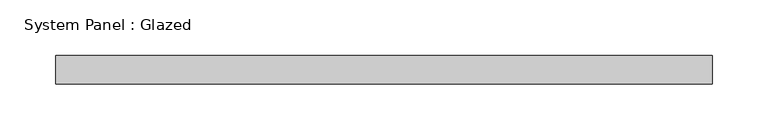
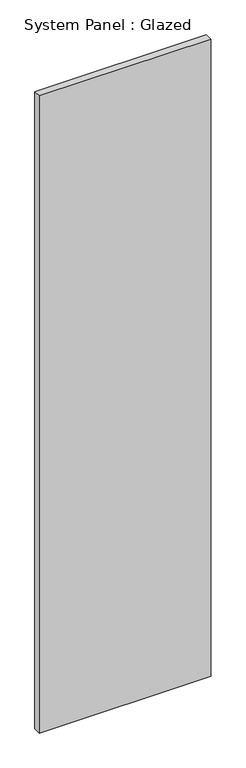
"""IFC4 building model written with IfcOpenShell, lengths in millimetres: plate geometry, System Panel : Glazed."""

from ifc_helpers import new_model, si_unit, origin, origin_with_axes, place, context, project, spatial, polyline, outline, extrude, source, transform, mapped, element, save


def system_panel_glazed_348cf8e9(model_context):
    return source(origin(), model_context, "Body", "SweptSolid", [
        extrude(outline(polyline([(294.2166666, 19.05), (-294.2166666, 19.05), (-294.2166666, 44.45), (294.2166666, 44.45), (294.2166666, 19.05)])), origin_with_axes(), (0.0, 0.0, 1.0), 2311.4),
    ])


if __name__ == "__main__":
    model = new_model("IFC4")
    model_context = context("Model", 3, world=origin())
    ifc_project = project(units=[si_unit("LENGTHUNIT", "METRE", prefix="MILLI")], contexts=[model_context])
    site = spatial("IfcSite", under=ifc_project)
    building = spatial("IfcBuilding", under=site)
    placement = place(None, origin())
    system_panel_glazed_shape = system_panel_glazed_348cf8e9(model_context)
    element("IfcPlate", 1, ObjectType="System Panel : Glazed", at=placement, inside=building, context=model_context, shape_type="MappedRepresentation", body=[
        mapped(system_panel_glazed_shape, transform((0.0, 0.0, 0.0), x_axis=(1.0, 0.0, 0.0), y_axis=(0.0, 1.0, 0.0), z_axis=(0.0, 0.0, 1.0))),
    ])
    save(model, "model.ifc")

# Revit data of these elements
# Type "System Panel : Glazed"
#   Construction Type Id = "GSP4R"
#   Analytic Construction = "1/8 in Pilkington single glazing"
#   Visual Light Transmittance = 0.9
#   Solar Heat Gain Coefficient = 0.86
#   Heat Transfer Coefficient (U) = 1.18115 BTU/(h·ft²·°F)
#   Define Thermal Properties by = 1
# Element 1 (IfcPlate, "System Panel : Glazed")
#   Materials on its faces: "Glass"
# Materials
#   "Glass": class "Glass", colour RGB 0 128 192, transparency 0.75, Description = "Soda Lime Glass", Cost = 0
